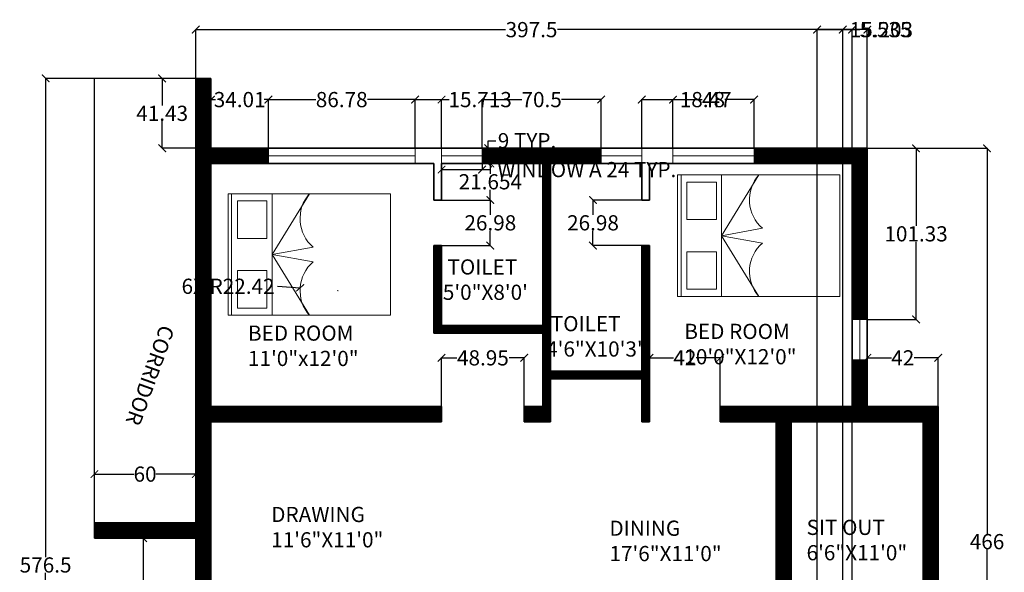
# Model space of a CAD drawing. Units: inches. Extents: x -124 to 468, y -83 to 563.
# Tile 3 of 3: x -124 to 459, y 235 to 563. Entities that reach past the tile are written whole.
import ezdxf

# ---------------------------------------------------------------- set-up
doc = ezdxf.new("R2010")
doc.units = ezdxf.units.IN
doc.header["$MEASUREMENT"] = 0
for name, color, linetype, lineweight in [('A-ANNO-DIMS', 2, 'Continuous', 18), ('A-AREA-IDEN', 7, 'Continuous', 18), ('A-FLOR', 8, 'Continuous', 25)]:
    doc.layers.add(name, color=color, linetype=linetype, lineweight=lineweight)
for name, color, linetype, lineweight, true_color in [('A-FURN', 37, 'Continuous', 18, 0x7c5b46), ('A-GLAZ', 145, 'Continuous', 18, 0x2a88b7), ('A-WALL', 149, 'Continuous', 35, 0x414448), ('A-WALL-PATT', 251, 'Continuous', 13, 0x585a5e)]:
    doc.layers.add(name, color=color, linetype=linetype, lineweight=lineweight, true_color=true_color)
doc.styles.get("Standard").update_dxf_attribs({"font": 'arial.ttf'})
doc.dimstyles.get("Standard").update_dxf_attribs({"dimtxt": 9, "dimasz": 4.5, "dimexe": 0.18, "dimexo": 0.0625, "dimgap": 0.09, "dimtad": 0, "dimtih": 1, "dimtoh": 1, "dimdec": 1, "dimzin": 0, "dimdsep": 46, "dimlunit": 4, "dimtxsty": 'Standard', "dimblk": 'ARCHTICK', "dimcen": 0.09, "dimadec": 0, "dimazin": 0, "dimtfac": 1, "dimtdec": 1, "dimtofl": 0, "dimtmove": 0, "dimatfit": 3, "dimfxl": 1, "dimtolj": 1, "dimtzin": 0, "dimarcsym": 0})

# ---------------------------------------------------------------- blocks, each defined once
blk = doc.blocks.new('BED-DOUBLE')
for p, q in [((0, 0), (0, 72)), ((0, 72), (96, 72)), ((2, 0), (2, 72)), ((26, 0), (26, 72)), ((48, 72), (26, 36)), ((96, 72), (96, 0)), ((26, 36), (50.21, 40.36)), ((26, 36), (48, 0)), ((26, 36), (50.21, 31.64)), ((50.21, 31.64), (26, 36)), ((96, 0), (0, 0))]:
    blk.add_line(p, q)
for points in [[(5.47, 67.74), (5.47, 45.52), (22.92, 45.52), (22.92, 67.74)], [(5.47, 4.26), (5.47, 26.48), (22.92, 26.48), (22.92, 4.26)]]:
    blk.add_lwpolyline(points, close=True)
for centre, start, end in [((64.91, 57.28), 138.97274, 229.00257), ((64.91, 14.72), 130.99743, 221.02726)]:
    blk.add_arc(centre, 22.42, start, end)
blk = doc.blocks.new('WIN-24IN')
for p, q in [((0, 0), (0, 9)), ((24, 0), (24, 9)), ((0, 4.5), (24, 4.5))]:
    blk.add_line(p, q)
blk = doc.blocks.new('_ArchTick')
at = {"color": 0, "linetype": 'ByBlock', "const_width": 0.15}
blk.add_lwpolyline([(-0.5, -0.5), (0.5, 0.5)], dxfattribs=at)
blk = doc.blocks.new('*D8')
at = {"layer": 'A-ANNO-DIMS', "color": 0, "lineweight": -2, "transparency": 16777216}
for p, q in [((125.98, 477.33), (125.98, 473.61)), ((125.98, 473.79), (149.98, 473.79)), ((149.98, 477.33), (149.98, 473.61)), ((149.98, 473.79), (154.48, 473.79))]:
    blk.add_line(p, q, dxfattribs=at)
at = {"layer": 'Defpoints', "color": 0, "transparency": 16777216}
for p in [(125.98, 477.39), (149.98, 477.39), (149.98, 473.79)]:
    blk.add_point(p, dxfattribs=at)
at = {"layer": 'A-ANNO-DIMS', "color": 0, "lineweight": -2, "transparency": 16777216, "xscale": 4.5, "yscale": 4.5, "zscale": 4.5, "rotation": 180}
blk.add_blockref('_ArchTick', (125.98, 473.79), dxfattribs=at)
at = {"layer": 'A-ANNO-DIMS', "color": 0, "lineweight": -2, "transparency": 16777216, "xscale": 4.5, "yscale": 4.5, "zscale": 4.5}
blk.add_blockref('_ArchTick', (149.98, 473.79), dxfattribs=at)
at = {"layer": 'A-ANNO-DIMS', "color": 0, "transparency": 16777216, "insert": (211.92, 473.79), "char_height": 9, "attachment_point": 5}
blk.add_mtext('\\A1;WINDOW A 24 TYP.', dxfattribs=at)
blk = doc.blocks.new('*D9')
at = {"layer": 'A-ANNO-DIMS', "color": 0, "lineweight": -2, "transparency": 16777216}
for p, q in [((153.58, 486.39), (153.58, 490.89)), ((153.58, 490.89), (158.08, 490.89)), ((150.04, 486.39), (153.76, 486.39)), ((153.58, 477.39), (153.58, 486.39)), ((150.04, 477.39), (153.76, 477.39))]:
    blk.add_line(p, q, dxfattribs=at)
at = {"layer": 'Defpoints', "color": 0, "transparency": 16777216}
for p in [(149.98, 486.39), (153.58, 486.39), (149.98, 477.39)]:
    blk.add_point(p, dxfattribs=at)
at = {"layer": 'A-ANNO-DIMS', "color": 0, "lineweight": -2, "transparency": 16777216, "xscale": 4.5, "yscale": 4.5, "zscale": 4.5}
for p, rotation in [((153.58, 486.39), 90), ((153.58, 477.39), 270)]:
    blk.add_blockref('_ArchTick', p, dxfattribs=dict(at, rotation=rotation))
at = {"layer": 'A-ANNO-DIMS', "color": 0, "transparency": 16777216, "insert": (176.57, 490.89), "char_height": 9, "attachment_point": 5}
blk.add_mtext('\\A1;9 TYP.', dxfattribs=at)
blk = doc.blocks.new('*D15')
at = {"layer": 'A-ANNO-DIMS', "color": 0, "lineweight": -2, "transparency": 16777216}
for p, q in [((-19.59, 527.82), (-108.57, 527.82)), ((-108.39, 527.82), (-108.39, 244.25)), ((-108.39, -48.69), (-108.39, 234.88)), ((-19.59, -48.69), (-108.57, -48.69))]:
    blk.add_line(p, q, dxfattribs=at)
at = {"layer": 'Defpoints', "color": 0, "transparency": 16777216}
for p in [(-108.39, 527.82), (-19.52, 527.82), (-19.52, -48.69)]:
    blk.add_point(p, dxfattribs=at)
at = {"layer": 'A-ANNO-DIMS', "color": 0, "lineweight": -2, "transparency": 16777216, "xscale": 4.5, "yscale": 4.5, "zscale": 4.5}
for p, rotation in [((-108.39, 527.82), 90), ((-108.39, -48.69), 270)]:
    blk.add_blockref('_ArchTick', p, dxfattribs=dict(at, rotation=rotation))
at = {"layer": 'A-ANNO-DIMS', "color": 0, "transparency": 16777216, "insert": (-108.39, 239.57), "char_height": 9, "attachment_point": 5}
blk.add_mtext('\\A1;576.5', dxfattribs=at)
blk = doc.blocks.new('*D16')
at = {"layer": 'A-ANNO-DIMS', "color": 0, "lineweight": -2, "transparency": 16777216}
for p, q in [((-19.52, 527.89), (-19.52, 556.87)), ((-19.52, 556.69), (163.92, 556.69)), ((377.98, 556.69), (194.53, 556.69)), ((377.98, 486.46), (377.98, 556.87))]:
    blk.add_line(p, q, dxfattribs=at)
at = {"layer": 'Defpoints', "color": 0, "transparency": 16777216}
for p in [(377.98, 556.69), (-19.52, 527.82), (377.98, 486.39)]:
    blk.add_point(p, dxfattribs=at)
at = {"layer": 'A-ANNO-DIMS', "color": 0, "lineweight": -2, "transparency": 16777216, "xscale": 4.5, "yscale": 4.5, "zscale": 4.5, "rotation": 180}
blk.add_blockref('_ArchTick', (-19.52, 556.69), dxfattribs=at)
at = {"layer": 'A-ANNO-DIMS', "color": 0, "lineweight": -2, "transparency": 16777216, "xscale": 4.5, "yscale": 4.5, "zscale": 4.5}
blk.add_blockref('_ArchTick', (377.98, 556.69), dxfattribs=at)
at = {"layer": 'A-ANNO-DIMS', "color": 0, "transparency": 16777216, "insert": (179.23, 556.69), "char_height": 9, "attachment_point": 5}
blk.add_mtext('\\A1;397.5', dxfattribs=at)
blk = doc.blocks.new('*D17')
at = {"layer": 'A-ANNO-DIMS', "color": 0, "lineweight": -2, "transparency": 16777216}
for p, q in [((378.04, 486.39), (449.02, 486.39)), ((448.84, 486.39), (448.84, 258.08)), ((448.84, 20.39), (448.84, 248.71)), ((378.04, 20.39), (449.02, 20.39))]:
    blk.add_line(p, q, dxfattribs=at)
at = {"layer": 'Defpoints', "color": 0, "transparency": 16777216}
for p in [(377.98, 486.39), (448.84, 486.39), (377.98, 20.39)]:
    blk.add_point(p, dxfattribs=at)
at = {"layer": 'A-ANNO-DIMS', "color": 0, "lineweight": -2, "transparency": 16777216, "xscale": 4.5, "yscale": 4.5, "zscale": 4.5}
for p, rotation in [((448.84, 486.39), 90), ((448.84, 20.39), 270)]:
    blk.add_blockref('_ArchTick', p, dxfattribs=dict(at, rotation=rotation))
at = {"layer": 'A-ANNO-DIMS', "color": 0, "transparency": 16777216, "insert": (448.84, 253.39), "char_height": 9, "attachment_point": 5}
blk.add_mtext('\\A1;466', dxfattribs=at)
blk = doc.blocks.new('*D18')
at = {"layer": 'A-ANNO-DIMS', "color": 0, "lineweight": -2, "transparency": 16777216}
for p, q in [((-10.59, 527.82), (-39.57, 527.82)), ((-39.39, 527.82), (-39.39, 511.8)), ((-39.39, 486.39), (-39.39, 502.42)), ((-10.59, 486.39), (-39.57, 486.39))]:
    blk.add_line(p, q, dxfattribs=at)
at = {"layer": 'Defpoints', "color": 0, "transparency": 16777216}
for p in [(-39.39, 527.82), (-10.52, 527.82), (-10.52, 486.39)]:
    blk.add_point(p, dxfattribs=at)
at = {"layer": 'A-ANNO-DIMS', "color": 0, "lineweight": -2, "transparency": 16777216, "xscale": 4.5, "yscale": 4.5, "zscale": 4.5}
for p, rotation in [((-39.39, 527.82), 90), ((-39.39, 486.39), 270)]:
    blk.add_blockref('_ArchTick', p, dxfattribs=dict(at, rotation=rotation))
at = {"layer": 'A-ANNO-DIMS', "color": 0, "transparency": 16777216, "insert": (-39.39, 507.11), "char_height": 9, "attachment_point": 5}
blk.add_mtext('\\A1;41.43', dxfattribs=at)
blk = doc.blocks.new('*D19')
at = {"layer": 'A-ANNO-DIMS', "color": 0, "lineweight": -2, "transparency": 16777216}
for p, q in [((-79.52, 264.59), (-79.52, 293.57)), ((-79.52, 293.39), (-56.07, 293.39)), ((-19.52, 293.39), (-42.98, 293.39)), ((-19.52, 264.59), (-19.52, 293.57))]:
    blk.add_line(p, q, dxfattribs=at)
at = {"layer": 'Defpoints', "color": 0, "transparency": 16777216}
for p in [(-19.52, 293.39), (-79.52, 264.53), (-19.52, 264.53)]:
    blk.add_point(p, dxfattribs=at)
at = {"layer": 'A-ANNO-DIMS', "color": 0, "lineweight": -2, "transparency": 16777216, "xscale": 4.5, "yscale": 4.5, "zscale": 4.5, "rotation": 180}
blk.add_blockref('_ArchTick', (-79.52, 293.39), dxfattribs=at)
at = {"layer": 'A-ANNO-DIMS', "color": 0, "lineweight": -2, "transparency": 16777216, "xscale": 4.5, "yscale": 4.5, "zscale": 4.5}
blk.add_blockref('_ArchTick', (-19.52, 293.39), dxfattribs=at)
at = {"layer": 'A-ANNO-DIMS', "color": 0, "transparency": 16777216, "insert": (-49.52, 293.39), "char_height": 9, "attachment_point": 5}
blk.add_mtext('\\A1;60', dxfattribs=at)
blk = doc.blocks.new('*D20')
at = {"layer": 'A-ANNO-DIMS', "color": 0, "lineweight": -2, "transparency": 16777216}
for p, q in [((377.98, 333.46), (377.98, 362.44)), ((377.98, 362.26), (392.31, 362.26)), ((419.98, 362.26), (405.65, 362.26)), ((419.98, 333.46), (419.98, 362.44))]:
    blk.add_line(p, q, dxfattribs=at)
at = {"layer": 'Defpoints', "color": 0, "transparency": 16777216}
for p in [(419.98, 362.26), (377.98, 333.39), (419.98, 333.39)]:
    blk.add_point(p, dxfattribs=at)
at = {"layer": 'A-ANNO-DIMS', "color": 0, "lineweight": -2, "transparency": 16777216, "xscale": 4.5, "yscale": 4.5, "zscale": 4.5, "rotation": 180}
blk.add_blockref('_ArchTick', (377.98, 362.26), dxfattribs=at)
at = {"layer": 'A-ANNO-DIMS', "color": 0, "lineweight": -2, "transparency": 16777216, "xscale": 4.5, "yscale": 4.5, "zscale": 4.5}
blk.add_blockref('_ArchTick', (419.98, 362.26), dxfattribs=at)
at = {"layer": 'A-ANNO-DIMS', "color": 0, "transparency": 16777216, "insert": (398.98, 362.26), "char_height": 9, "attachment_point": 5}
blk.add_mtext('\\A1;42', dxfattribs=at)
blk = doc.blocks.new('*D22')
at = {"layer": 'A-ANNO-DIMS', "color": 0, "lineweight": -2, "transparency": 16777216}
for p, q in [((-10.52, 486.46), (-10.52, 515.44)), ((-10.52, 515.26), (-7.92, 515.26)), ((23.48, 515.26), (20.88, 515.26)), ((23.48, 486.46), (23.48, 515.44))]:
    blk.add_line(p, q, dxfattribs=at)
at = {"layer": 'Defpoints', "color": 0, "transparency": 16777216}
for p in [(23.48, 515.26), (-10.52, 486.39), (23.48, 486.39)]:
    blk.add_point(p, dxfattribs=at)
at = {"layer": 'A-ANNO-DIMS', "color": 0, "lineweight": -2, "transparency": 16777216, "xscale": 4.5, "yscale": 4.5, "zscale": 4.5, "rotation": 180}
blk.add_blockref('_ArchTick', (-10.52, 515.26), dxfattribs=at)
at = {"layer": 'A-ANNO-DIMS', "color": 0, "lineweight": -2, "transparency": 16777216, "xscale": 4.5, "yscale": 4.5, "zscale": 4.5}
blk.add_blockref('_ArchTick', (23.48, 515.26), dxfattribs=at)
at = {"layer": 'A-ANNO-DIMS', "color": 0, "transparency": 16777216, "insert": (6.48, 515.26), "char_height": 9, "attachment_point": 5}
blk.add_mtext('\\A1;34.01', dxfattribs=at)
blk = doc.blocks.new('*D23')
at = {"layer": 'A-ANNO-DIMS', "color": 0, "lineweight": -2, "transparency": 16777216}
for p, q in [((23.48, 486.46), (23.48, 515.44)), ((23.48, 515.26), (51.58, 515.26)), ((110.26, 515.26), (82.16, 515.26)), ((110.26, 486.46), (110.26, 515.44))]:
    blk.add_line(p, q, dxfattribs=at)
at = {"layer": 'Defpoints', "color": 0, "transparency": 16777216}
for p in [(110.26, 515.26), (23.48, 486.39), (110.26, 486.39)]:
    blk.add_point(p, dxfattribs=at)
at = {"layer": 'A-ANNO-DIMS', "color": 0, "lineweight": -2, "transparency": 16777216, "xscale": 4.5, "yscale": 4.5, "zscale": 4.5, "rotation": 180}
blk.add_blockref('_ArchTick', (23.48, 515.26), dxfattribs=at)
at = {"layer": 'A-ANNO-DIMS', "color": 0, "lineweight": -2, "transparency": 16777216, "xscale": 4.5, "yscale": 4.5, "zscale": 4.5}
blk.add_blockref('_ArchTick', (110.26, 515.26), dxfattribs=at)
at = {"layer": 'A-ANNO-DIMS', "color": 0, "transparency": 16777216, "insert": (66.87, 515.26), "char_height": 9, "attachment_point": 5}
blk.add_mtext('\\A1;86.78', dxfattribs=at)
blk = doc.blocks.new('*D24')
at = {"layer": 'A-ANNO-DIMS', "color": 0, "lineweight": -2, "transparency": 16777216}
for p, q in [((110.26, 486.46), (110.26, 515.44)), ((110.26, 515.26), (125.98, 515.26)), ((125.98, 486.46), (125.98, 515.44)), ((125.98, 515.26), (130.48, 515.26))]:
    blk.add_line(p, q, dxfattribs=at)
at = {"layer": 'Defpoints', "color": 0, "transparency": 16777216}
for p in [(125.98, 515.26), (110.26, 486.39), (125.98, 486.39)]:
    blk.add_point(p, dxfattribs=at)
at = {"layer": 'A-ANNO-DIMS', "color": 0, "lineweight": -2, "transparency": 16777216, "xscale": 4.5, "yscale": 4.5, "zscale": 4.5, "rotation": 180}
blk.add_blockref('_ArchTick', (110.26, 515.26), dxfattribs=at)
at = {"layer": 'A-ANNO-DIMS', "color": 0, "lineweight": -2, "transparency": 16777216, "xscale": 4.5, "yscale": 4.5, "zscale": 4.5}
blk.add_blockref('_ArchTick', (125.98, 515.26), dxfattribs=at)
at = {"layer": 'A-ANNO-DIMS', "color": 0, "transparency": 16777216, "insert": (148.82, 515.26), "char_height": 9, "attachment_point": 5}
blk.add_mtext('\\A1;15.713', dxfattribs=at)
blk = doc.blocks.new('*D25')
at = {"layer": 'A-ANNO-DIMS', "color": 0, "lineweight": -2, "transparency": 16777216}
for p, q in [((149.98, 486.46), (149.98, 515.44)), ((149.98, 515.26), (173.45, 515.26)), ((220.48, 515.26), (197, 515.26)), ((220.48, 486.46), (220.48, 515.44))]:
    blk.add_line(p, q, dxfattribs=at)
at = {"layer": 'Defpoints', "color": 0, "transparency": 16777216}
for p in [(220.48, 515.26), (149.98, 486.39), (220.48, 486.39)]:
    blk.add_point(p, dxfattribs=at)
at = {"layer": 'A-ANNO-DIMS', "color": 0, "lineweight": -2, "transparency": 16777216, "xscale": 4.5, "yscale": 4.5, "zscale": 4.5, "rotation": 180}
blk.add_blockref('_ArchTick', (149.98, 515.26), dxfattribs=at)
at = {"layer": 'A-ANNO-DIMS', "color": 0, "lineweight": -2, "transparency": 16777216, "xscale": 4.5, "yscale": 4.5, "zscale": 4.5}
blk.add_blockref('_ArchTick', (220.48, 515.26), dxfattribs=at)
at = {"layer": 'A-ANNO-DIMS', "color": 0, "transparency": 16777216, "insert": (185.23, 515.26), "char_height": 9, "attachment_point": 5}
blk.add_mtext('\\A1;70.5', dxfattribs=at)
blk = doc.blocks.new('*D26')
at = {"layer": 'A-ANNO-DIMS', "color": 0, "lineweight": -2, "transparency": 16777216}
for p, q in [((244.48, 486.46), (244.48, 515.44)), ((244.48, 515.26), (262.95, 515.26)), ((262.95, 486.46), (262.95, 515.44)), ((262.95, 515.26), (267.45, 515.26))]:
    blk.add_line(p, q, dxfattribs=at)
at = {"layer": 'Defpoints', "color": 0, "transparency": 16777216}
for p in [(262.95, 515.26), (244.48, 486.39), (262.95, 486.39)]:
    blk.add_point(p, dxfattribs=at)
at = {"layer": 'A-ANNO-DIMS', "color": 0, "lineweight": -2, "transparency": 16777216, "xscale": 4.5, "yscale": 4.5, "zscale": 4.5, "rotation": 180}
blk.add_blockref('_ArchTick', (244.48, 515.26), dxfattribs=at)
at = {"layer": 'A-ANNO-DIMS', "color": 0, "lineweight": -2, "transparency": 16777216, "xscale": 4.5, "yscale": 4.5, "zscale": 4.5}
blk.add_blockref('_ArchTick', (262.95, 515.26), dxfattribs=at)
at = {"layer": 'A-ANNO-DIMS', "color": 0, "transparency": 16777216, "insert": (282.3, 515.26), "char_height": 9, "attachment_point": 5}
blk.add_mtext('\\A1;18.47', dxfattribs=at)
blk = doc.blocks.new('*D27')
at = {"layer": 'A-ANNO-DIMS', "color": 0, "lineweight": -2, "transparency": 16777216}
for p, q in [((262.95, 486.46), (262.95, 515.44)), ((262.95, 515.26), (280.22, 515.26)), ((310.95, 515.26), (293.67, 515.26)), ((310.95, 486.46), (310.95, 515.44))]:
    blk.add_line(p, q, dxfattribs=at)
at = {"layer": 'Defpoints', "color": 0, "transparency": 16777216}
for p in [(310.95, 515.26), (262.95, 486.39), (310.95, 486.39)]:
    blk.add_point(p, dxfattribs=at)
at = {"layer": 'A-ANNO-DIMS', "color": 0, "lineweight": -2, "transparency": 16777216, "xscale": 4.5, "yscale": 4.5, "zscale": 4.5, "rotation": 180}
blk.add_blockref('_ArchTick', (262.95, 515.26), dxfattribs=at)
at = {"layer": 'A-ANNO-DIMS', "color": 0, "lineweight": -2, "transparency": 16777216, "xscale": 4.5, "yscale": 4.5, "zscale": 4.5}
blk.add_blockref('_ArchTick', (310.95, 515.26), dxfattribs=at)
at = {"layer": 'A-ANNO-DIMS', "color": 0, "transparency": 16777216, "insert": (286.95, 515.26), "char_height": 9, "attachment_point": 5}
blk.add_mtext('\\A1;48', dxfattribs=at)
blk = doc.blocks.new('*D33')
at = {"layer": 'A-ANNO-DIMS', "color": 0, "lineweight": -2, "transparency": 16777216}
for p, q in [((378.04, 486.39), (407.02, 486.39)), ((406.84, 486.39), (406.84, 440.42)), ((406.84, 385.07), (406.84, 431.04)), ((378.04, 385.07), (407.02, 385.07))]:
    blk.add_line(p, q, dxfattribs=at)
at = {"layer": 'Defpoints', "color": 0, "transparency": 16777216}
for p in [(377.98, 486.39), (377.98, 385.07), (406.84, 385.07)]:
    blk.add_point(p, dxfattribs=at)
at = {"layer": 'A-ANNO-DIMS', "color": 0, "lineweight": -2, "transparency": 16777216, "xscale": 4.5, "yscale": 4.5, "zscale": 4.5}
for p, rotation in [((406.84, 486.39), 90), ((406.84, 385.07), 270)]:
    blk.add_blockref('_ArchTick', p, dxfattribs=dict(at, rotation=rotation))
at = {"layer": 'A-ANNO-DIMS', "color": 0, "transparency": 16777216, "insert": (406.84, 435.73), "char_height": 9, "attachment_point": 5}
blk.add_mtext('\\A1;101.33', dxfattribs=at)
blk = doc.blocks.new('*D36')
at = {"layer": 'A-ANNO-DIMS', "color": 0, "lineweight": -2, "transparency": 16777216}
for p, q in [((-79.46, 255.53), (-50.48, 255.53)), ((-50.66, 255.53), (-50.66, 210.64)), ((-50.66, 156.37), (-50.66, 201.27)), ((-79.46, 156.37), (-50.48, 156.37))]:
    blk.add_line(p, q, dxfattribs=at)
at = {"layer": 'Defpoints', "color": 0, "transparency": 16777216}
for p in [(-79.52, 255.53), (-79.52, 156.37), (-50.66, 156.37)]:
    blk.add_point(p, dxfattribs=at)
at = {"layer": 'A-ANNO-DIMS', "color": 0, "lineweight": -2, "transparency": 16777216, "xscale": 4.5, "yscale": 4.5, "zscale": 4.5}
for p, rotation in [((-50.66, 255.53), 90), ((-50.66, 156.37), 270)]:
    blk.add_blockref('_ArchTick', p, dxfattribs=dict(at, rotation=rotation))
at = {"layer": 'A-ANNO-DIMS', "color": 0, "transparency": 16777216, "insert": (-50.66, 205.95), "char_height": 9, "attachment_point": 5}
blk.add_mtext('\\A1;99.15', dxfattribs=at)
blk = doc.blocks.new('*D38')
at = {"layer": 'A-ANNO-DIMS', "color": 0, "lineweight": -2, "transparency": 16777216}
for p, q in [((125.98, 333.46), (125.98, 362.44)), ((125.98, 362.26), (134.96, 362.26)), ((174.93, 362.26), (165.94, 362.26)), ((174.93, 333.46), (174.93, 362.44))]:
    blk.add_line(p, q, dxfattribs=at)
at = {"layer": 'Defpoints', "color": 0, "transparency": 16777216}
for p in [(174.93, 362.26), (125.98, 333.39), (174.93, 333.39)]:
    blk.add_point(p, dxfattribs=at)
at = {"layer": 'A-ANNO-DIMS', "color": 0, "lineweight": -2, "transparency": 16777216, "xscale": 4.5, "yscale": 4.5, "zscale": 4.5, "rotation": 180}
blk.add_blockref('_ArchTick', (125.98, 362.26), dxfattribs=at)
at = {"layer": 'A-ANNO-DIMS', "color": 0, "lineweight": -2, "transparency": 16777216, "xscale": 4.5, "yscale": 4.5, "zscale": 4.5}
blk.add_blockref('_ArchTick', (174.93, 362.26), dxfattribs=at)
at = {"layer": 'A-ANNO-DIMS', "color": 0, "transparency": 16777216, "insert": (150.45, 362.26), "char_height": 9, "attachment_point": 5}
blk.add_mtext('\\A1;48.95', dxfattribs=at)
blk = doc.blocks.new('*D39')
at = {"layer": 'A-ANNO-DIMS', "color": 0, "lineweight": -2, "transparency": 16777216}
for p, q in [((248.98, 333.46), (248.98, 362.44)), ((248.98, 362.26), (263.31, 362.26)), ((290.98, 362.26), (276.65, 362.26)), ((290.98, 333.46), (290.98, 362.44))]:
    blk.add_line(p, q, dxfattribs=at)
at = {"layer": 'Defpoints', "color": 0, "transparency": 16777216}
for p in [(290.98, 362.26), (248.98, 333.39), (290.98, 333.39)]:
    blk.add_point(p, dxfattribs=at)
at = {"layer": 'A-ANNO-DIMS', "color": 0, "lineweight": -2, "transparency": 16777216, "xscale": 4.5, "yscale": 4.5, "zscale": 4.5, "rotation": 180}
blk.add_blockref('_ArchTick', (248.98, 362.26), dxfattribs=at)
at = {"layer": 'A-ANNO-DIMS', "color": 0, "lineweight": -2, "transparency": 16777216, "xscale": 4.5, "yscale": 4.5, "zscale": 4.5}
blk.add_blockref('_ArchTick', (290.98, 362.26), dxfattribs=at)
at = {"layer": 'A-ANNO-DIMS', "color": 0, "transparency": 16777216, "insert": (269.98, 362.26), "char_height": 9, "attachment_point": 5}
blk.add_mtext('\\A1;42', dxfattribs=at)
blk = doc.blocks.new('*D42')
at = {"layer": 'A-ANNO-DIMS', "color": 0, "lineweight": -2, "transparency": 16777216}
for p, q in [((126.04, 455.74), (155.02, 455.74)), ((154.84, 455.74), (154.84, 446.93)), ((154.84, 428.76), (154.84, 437.56)), ((126.04, 428.76), (155.02, 428.76))]:
    blk.add_line(p, q, dxfattribs=at)
at = {"layer": 'Defpoints', "color": 0, "transparency": 16777216}
for p in [(125.98, 455.74), (125.98, 428.76), (154.84, 428.76)]:
    blk.add_point(p, dxfattribs=at)
at = {"layer": 'A-ANNO-DIMS', "color": 0, "lineweight": -2, "transparency": 16777216, "xscale": 4.5, "yscale": 4.5, "zscale": 4.5}
for p, rotation in [((154.84, 455.74), 90), ((154.84, 428.76), 270)]:
    blk.add_blockref('_ArchTick', p, dxfattribs=dict(at, rotation=rotation))
at = {"layer": 'A-ANNO-DIMS', "color": 0, "transparency": 16777216, "insert": (154.84, 442.25), "char_height": 9, "attachment_point": 5}
blk.add_mtext('\\A1;26.98', dxfattribs=at)
blk = doc.blocks.new('*D43')
at = {"layer": 'A-ANNO-DIMS', "color": 0, "lineweight": -2, "transparency": 16777216}
for p, q in [((244.41, 455.74), (215.43, 455.74)), ((215.61, 455.74), (215.61, 446.93)), ((215.61, 428.76), (215.61, 437.56)), ((244.41, 428.76), (215.43, 428.76))]:
    blk.add_line(p, q, dxfattribs=at)
at = {"layer": 'Defpoints', "color": 0, "transparency": 16777216}
for p in [(215.61, 455.74), (244.48, 455.74), (244.48, 428.76)]:
    blk.add_point(p, dxfattribs=at)
at = {"layer": 'A-ANNO-DIMS', "color": 0, "lineweight": -2, "transparency": 16777216, "xscale": 4.5, "yscale": 4.5, "zscale": 4.5}
for p, rotation in [((215.61, 455.74), 90), ((215.61, 428.76), 270)]:
    blk.add_blockref('_ArchTick', p, dxfattribs=dict(at, rotation=rotation))
at = {"layer": 'A-ANNO-DIMS', "color": 0, "transparency": 16777216, "insert": (215.61, 442.25), "char_height": 9, "attachment_point": 5}
blk.add_mtext('\\A1;26.98', dxfattribs=at)
blk = doc.blocks.new('*D44')
at = {"layer": 'A-ANNO-DIMS', "color": 0, "lineweight": -2, "transparency": 16777216}
for p, q in [((126.04, 477.39), (155.02, 477.39)), ((154.84, 477.39), (154.84, 471.25)), ((154.84, 455.74), (154.84, 461.88)), ((126.04, 455.74), (155.02, 455.74))]:
    blk.add_line(p, q, dxfattribs=at)
at = {"layer": 'Defpoints', "color": 0, "transparency": 16777216}
for p in [(125.98, 477.39), (125.98, 455.74), (154.84, 455.74)]:
    blk.add_point(p, dxfattribs=at)
at = {"layer": 'A-ANNO-DIMS', "color": 0, "lineweight": -2, "transparency": 16777216, "xscale": 4.5, "yscale": 4.5, "zscale": 4.5}
for p, rotation in [((154.84, 477.39), 90), ((154.84, 455.74), 270)]:
    blk.add_blockref('_ArchTick', p, dxfattribs=dict(at, rotation=rotation))
at = {"layer": 'A-ANNO-DIMS', "color": 0, "transparency": 16777216, "insert": (154.84, 466.57), "char_height": 9, "attachment_point": 5}
blk.add_mtext('\\A1;21.654', dxfattribs=at)
blk = doc.blocks.new('*D56')
at = {"layer": 'A-ANNO-DIMS', "color": 0, "lineweight": -2, "transparency": 16777216}
for p, q in [((348.24, 156.86), (348.24, 556.87)), ((348.24, 556.69), (363.44, 556.69)), ((363.44, 156.86), (363.44, 556.87)), ((363.44, 556.69), (367.94, 556.69))]:
    blk.add_line(p, q, dxfattribs=at)
at = {"layer": 'Defpoints', "color": 0, "transparency": 16777216}
for p in [(363.44, 556.69), (348.24, 156.8), (363.44, 156.8)]:
    blk.add_point(p, dxfattribs=at)
at = {"layer": 'A-ANNO-DIMS', "color": 0, "lineweight": -2, "transparency": 16777216, "xscale": 4.5, "yscale": 4.5, "zscale": 4.5, "rotation": 180}
blk.add_blockref('_ArchTick', (348.24, 556.69), dxfattribs=at)
at = {"layer": 'A-ANNO-DIMS', "color": 0, "lineweight": -2, "transparency": 16777216, "xscale": 4.5, "yscale": 4.5, "zscale": 4.5}
blk.add_blockref('_ArchTick', (363.44, 556.69), dxfattribs=at)
at = {"layer": 'A-ANNO-DIMS', "color": 0, "transparency": 16777216, "insert": (386.29, 556.69), "char_height": 9, "attachment_point": 5}
blk.add_mtext('\\A1;15.203', dxfattribs=at)
blk = doc.blocks.new('*D59')
at = {"layer": 'A-ANNO-DIMS', "color": 0, "lineweight": -2, "transparency": 16777216}
for p, q in [((363.44, 156.86), (363.44, 556.87)), ((363.44, 556.69), (368.98, 556.69)), ((368.98, 183.46), (368.98, 556.87)), ((368.98, 556.69), (373.48, 556.69))]:
    blk.add_line(p, q, dxfattribs=at)
at = {"layer": 'Defpoints', "color": 0, "transparency": 16777216}
for p in [(368.98, 556.69), (368.98, 183.39), (363.44, 156.8)]:
    blk.add_point(p, dxfattribs=at)
at = {"layer": 'A-ANNO-DIMS', "color": 0, "lineweight": -2, "transparency": 16777216, "xscale": 4.5, "yscale": 4.5, "zscale": 4.5, "rotation": 180}
blk.add_blockref('_ArchTick', (363.44, 556.69), dxfattribs=at)
at = {"layer": 'A-ANNO-DIMS', "color": 0, "lineweight": -2, "transparency": 16777216, "xscale": 4.5, "yscale": 4.5, "zscale": 4.5}
blk.add_blockref('_ArchTick', (368.98, 556.69), dxfattribs=at)
at = {"layer": 'A-ANNO-DIMS', "color": 0, "transparency": 16777216, "insert": (388.79, 556.69), "char_height": 9, "attachment_point": 5}
blk.add_mtext('\\A1;5.535', dxfattribs=at)
blk = doc.blocks.new('*D62')
at = {"layer": 'A-ANNO-DIMS', "color": 0, "lineweight": -2, "transparency": 16777216}
for p, q in [((28.84, 404.66), (42.26, 403.73)), ((64.54, 402.17), (64.72, 402.17)), ((64.63, 402.08), (64.63, 402.26))]:
    blk.add_line(p, q, dxfattribs=at)
at = {"layer": 'Defpoints', "color": 0, "transparency": 16777216}
for p in [(42.26, 403.73), (64.63, 402.17)]:
    blk.add_point(p, dxfattribs=at)
at = {"layer": 'A-ANNO-DIMS', "color": 0, "lineweight": -2, "transparency": 16777216, "xscale": 4.5, "yscale": 4.5, "zscale": 4.5, "rotation": 356.0116510722241}
blk.add_blockref('_ArchTick', (42.26, 403.73), dxfattribs=at)
at = {"layer": 'A-ANNO-DIMS', "color": 0, "transparency": 16777216, "insert": (-0.39, 404.66), "char_height": 9, "attachment_point": 5}
blk.add_mtext('\\A1;6X R22.42', dxfattribs=at)

msp = doc.modelspace()

# ---------------------------------------------------------------- hatches: boundary and pattern name
at = {"layer": 'A-WALL-PATT'}
h = msp.add_hatch(dxfattribs=at)
h.set_pattern_fill('ANSI31', color=256)
h.set_pattern_definition([(45, (-392.07623, 0), (-0.088388348, 0.088388348), [])])
h.paths.add_polyline_path([(377.9763, 141.7862), (377.9763, 183.3929), (419.9763, 183.3929), (419.9763, 192.3929), (419.9763, 324.3929), (419.9763, 333.3929), (377.9763, 333.3929), (377.9763, 361.0673), (368.9763, 361.0673), (368.9763, 333.3929), (290.9763, 333.3929), (290.9763, 324.3929), (323.9763, 324.3929), (323.9763, 192.3929), (323.9763, 183.3929), (368.9763, 183.3929), (368.9763, 141.7862), (368.9763, 29.3929), (343.3064, 29.3929), (343.3064, 20.3929), (377.9763, 20.3929)])
h.paths.add_polyline_path([(368.9763, 192.3929), (332.9763, 192.3929), (332.9763, 324.3929), (368.9763, 324.3929), (410.9763, 324.3929), (410.9763, 192.3929)], flags=16)
h.paths.add_polyline_path([(215.9763, 29.3929), (179.9763, 29.3929), (179.9763, 75.2245), (175.4763, 75.2245), (175.4763, 29.3929), (167.489, 29.3929), (167.489, 20.3929), (215.9763, 20.3929)])
h.paths.add_polyline_path([(266.8777, 29.3929), (244.4763, 29.3929), (244.4763, 141.7862), (244.4763, 183.3929), (257.421, 183.3929), (257.421, 192.3929), (170.9763, 192.3929), (170.9763, 183.3929), (175.4763, 183.3929), (175.4763, 141.7862), (175.4763, 106.8322), (179.9763, 106.8322), (179.9763, 141.7862), (179.9763, 183.3929), (239.9763, 183.3929), (239.9763, 141.7862), (239.9763, 29.3929), (239.9763, 20.3929), (266.8777, 20.3929)])
h.paths.add_polyline_path([(131.489, 29.3929), (62.8565, 29.3929), (62.8565, 20.3929), (131.489, 20.3929)])
h.paths.add_polyline_path([(26.8565, 29.3929), (-10.5237, 29.3929), (-10.5237, 141.7862), (-10.5237, 183.3929), (125.9763, 183.3929), (125.9763, 192.3929), (-10.5237, 192.3929), (-10.5237, 324.3929), (125.9763, 324.3929), (125.9763, 333.3929), (-10.5237, 333.3929), (-10.5237, 477.3929), (23.4837, 477.3929), (23.4837, 486.3929), (-10.5237, 486.3929), (-10.5237, 527.8228), (-19.5237, 527.8228), (-19.5237, 486.3929), (-19.5237, 264.528), (-79.5237, 264.528), (-79.5237, 255.528), (-19.5237, 255.528), (-19.5237, 156.3747), (-79.5237, 156.3747), (-79.5237, 147.3747), (-19.5237, 147.3747), (-19.5237, 141.7862), (-19.5237, -48.6869), (-10.5237, -48.6869), (-10.5237, 20.3929), (26.8565, 20.3929)])
h.paths.add_polyline_path([(220.4763, 486.3929), (149.9763, 486.3929), (149.9763, 477.3929), (185.9763, 477.3929), (185.9763, 381.3929), (125.9763, 381.3929), (125.9763, 428.759), (121.4763, 428.759), (121.4763, 376.8929), (125.9763, 376.8929), (185.9763, 376.8929), (185.9763, 333.3929), (174.9252, 333.3929), (174.9252, 324.3929), (190.4763, 324.3929), (190.4763, 333.3929), (190.4763, 349.8929), (244.4763, 349.8929), (244.4763, 333.3929), (244.4763, 324.3929), (248.9763, 324.3929), (248.9763, 333.3929), (248.9763, 428.759), (244.4763, 428.759), (244.4763, 354.3929), (190.4763, 354.3929), (190.4763, 477.3929), (220.4763, 477.3929)])
h.paths.add_polyline_path([(377.9763, 486.3929), (310.948, 486.3929), (310.948, 477.3929), (368.9763, 477.3929), (368.9763, 385.0673), (377.9763, 385.0673)])
h.paths.add_polyline_path([(339.1974, 237.2234), (400.8652, 237.2234), (400.8652, 270.8067), (339.1974, 270.8067)], flags=8)
h.paths.add_polyline_path([(182.8614, 357.8948), (247.9303, 357.8948), (247.9303, 391.478), (182.8614, 391.478)], flags=25)

# ---------------------------------------------------------------- linework, layer by layer
at = {"layer": 'A-FLOR'}
for p in [(-79.5237, 264.528), (-19.5237, 527.8228)]:
    msp.add_line(p, (-79.5237, 527.8228), dxfattribs=at)
at = {"layer": 'A-GLAZ'}
for p, q in [((23.4837, 486.3929), (23.4837, 477.3929)), ((110.2629, 486.3929), (110.2629, 477.3929)), ((262.948, 486.3929), (262.948, 477.3929)), ((310.948, 486.3929), (310.948, 477.3929)), ((23.4837, 481.8929), (110.2629, 481.8929)), ((262.948, 481.8929), (310.948, 481.8929))]:
    msp.add_line(p, q, dxfattribs=at)
at = {"layer": 'A-WALL'}
for p, q in [((-19.5237, 486.3929), (-19.5237, 527.8228)), ((-19.5237, 527.8228), (-10.5237, 527.8228)), ((-10.5237, 486.3929), (-10.5237, 527.8228)), ((-19.5237, 486.3929), (-19.5237, 264.528)), ((-10.5237, 486.3929), (377.9763, 486.3929)), ((377.9763, 486.3929), (377.9763, 333.3929)), ((-10.5237, 477.3929), (-10.5237, 333.3929)), ((-10.5237, 477.3929), (121.4763, 477.3929)), ((121.4763, 477.3929), (121.4763, 455.7385)), ((125.9763, 477.3929), (125.9763, 455.7385)), ((125.9763, 477.3929), (185.9763, 477.3929)), ((185.9763, 477.3929), (185.9763, 381.3929)), ((190.4763, 477.3929), (190.4763, 354.3929)), ((190.4763, 477.3929), (244.4763, 477.3929)), ((244.4763, 477.3929), (244.4763, 455.7385)), ((248.9763, 477.3929), (248.9763, 455.7385)), ((248.9763, 477.3929), (368.9763, 477.3929)), ((368.9763, 477.3929), (368.9763, 333.3929)), ((125.9763, 455.7385), (121.4763, 455.7385)), ((244.4763, 455.7385), (248.9763, 455.7385)), ((121.4763, 428.759), (121.4763, 376.8929)), ((125.9763, 428.759), (121.4763, 428.759)), ((125.9763, 428.759), (125.9763, 381.3929)), ((244.4763, 428.759), (248.9763, 428.759)), ((244.4763, 428.759), (244.4763, 354.3929)), ((248.9763, 428.759), (248.9763, 333.3929)), ((125.9763, 381.3929), (185.9763, 381.3929)), ((125.9763, 376.8929), (121.4763, 376.8929)), ((125.9763, 376.8929), (185.9763, 376.8929)), ((185.9763, 376.8929), (185.9763, 333.3929)), ((190.4763, 354.3929), (244.4763, 354.3929)), ((190.4763, 349.8929), (244.4763, 349.8929)), ((190.4763, 349.8929), (190.4763, 333.3929)), ((244.4763, 349.8929), (244.4763, 333.3929)), ((-10.5237, 333.3929), (125.9763, 333.3929)), ((125.9763, 333.3929), (125.9763, 324.3929)), ((174.9252, 333.3929), (174.9252, 324.3929)), ((174.9252, 333.3929), (185.9763, 333.3929)), ((190.4763, 333.3929), (190.4763, 324.3929)), ((244.4763, 333.3929), (244.4763, 324.3929)), ((248.9763, 333.3929), (248.9763, 324.3929)), ((290.9763, 333.3929), (368.9763, 333.3929)), ((290.9763, 333.3929), (290.9763, 324.3929)), ((377.9763, 333.3929), (419.9763, 333.3929)), ((419.9763, 324.3929), (419.9763, 333.3929)), ((-10.5237, 324.3929), (125.9763, 324.3929)), ((-10.5237, 324.3929), (-10.5237, 192.3929)), ((174.9252, 324.3929), (190.4763, 324.3929)), ((244.4763, 324.3929), (248.9763, 324.3929)), ((290.9763, 324.3929), (323.9763, 324.3929)), ((323.9763, 324.3929), (323.9763, 192.3929)), ((332.9763, 324.3929), (332.9763, 192.3929)), ((332.9763, 324.3929), (368.9763, 324.3929)), ((368.9763, 324.3929), (410.9763, 324.3929)), ((410.9763, 324.3929), (410.9763, 192.3929)), ((419.9763, 324.3929), (419.9763, 192.3929)), ((-79.5237, 264.528), (-79.5237, 255.528)), ((-79.5237, 264.528), (-19.5237, 264.528)), ((-79.5237, 255.528), (-19.5237, 255.528)), ((-19.5237, 255.528), (-19.5237, 156.3747))]:
    msp.add_line(p, q, dxfattribs=at)

# ---------------------------------------------------------------- block references
at = {"layer": 'A-FURN'}
for p in [(265.7059, 398.6343), (-0.286, 387.451)]:
    msp.add_blockref('BED-DOUBLE', p, dxfattribs=at)
at = {"layer": 'A-GLAZ'}
msp.add_blockref('WIN-24IN', (125.976, 477.393), dxfattribs=at)
for p, rotation in [((244.4766, 486.3927), 180), ((368.9764, 385.0676), 269.9999999999998)]:
    msp.add_blockref('WIN-24IN', p, dxfattribs=dict(at, rotation=rotation))

# ---------------------------------------------------------------- texts
at = {"layer": 'A-AREA-IDEN', "char_height": 9, "attachment_point": 1}
for s, insert in [('  TOILET\\P 5\'0"X8\'0\'', (123.9812, 420.6103)), ('  TOILET\\P 4\'6"X10\'3"', (185.1114, 387.0056)), ('BED ROOM\\P11\'0"x12\'0"', (11.3998, 381.4049)), ('BED ROOM\\P10\'0"X12\'0"', (269.6748, 382.4232)), ('DRAWING\\P11\'6"X11\'0"', (25.1541, 273.9717)), ('DINING\\P17\'6"X11\'0"', (225.3554, 265.8251)), ('SIT OUT\\P6\'6"X11\'0"', (342.0122, 266.3343))]:
    msp.add_mtext_dynamic_manual_height_columns(s, width=177.374172, gutter_width=1, heights=[0], dxfattribs=dict(at, insert=insert))
at = {"layer": 'A-AREA-IDEN', "insert": (-31.8995, 379.3341), "char_height": 9, "attachment_point": 1, "rotation": 250.244164}
msp.add_mtext_dynamic_manual_height_columns('CORRIDOR', width=177.374172, gutter_width=1, heights=[0], dxfattribs=at)

# ---------------------------------------------------------------- dimensions: what is measured, and where the dimension line sits
at = {"layer": 'A-ANNO-DIMS'}
for base, p1, p2, override, picture, middle in [((377.9763, 556.6878), (-19.5237, 527.8228), (377.9763, 486.3929), {"dimdec": 1, "dimlfac": 1, "dimrnd": 0, "dimzin": 0, "dimdsep": 46, "dimlunit": 2}, '*D16', (179.2263, 556.6878)), ((363.4417, 556.6878), (348.2388, 156.7996), (363.4417, 156.7996), {"dimdec": 3, "dimlfac": 1, "dimrnd": 0, "dimzin": 0, "dimdsep": 46, "dimlunit": 2}, '*D56', (386.2895, 556.6878)), ((368.9763, 556.6878), (363.4417, 156.7996), (368.9763, 183.3929), {"dimdec": 3, "dimlfac": 1, "dimrnd": 0, "dimzin": 0, "dimdsep": 46, "dimlunit": 2}, '*D59', (388.7853, 556.6878)), ((23.4837, 515.2579), (-10.5237, 486.3929), (23.4837, 486.3929), {"dimdec": 2, "dimlfac": 1, "dimrnd": 0, "dimzin": 0, "dimdsep": 46, "dimlunit": 2}, '*D22', (6.48, 515.2579)), ((110.2629, 515.2579), (23.4837, 486.3929), (110.2629, 486.3929), {"dimdec": 2, "dimlfac": 1, "dimrnd": 0, "dimzin": 0, "dimdsep": 46, "dimlunit": 2}, '*D23', (66.8733, 515.2579)), ((220.4763, 515.2579), (149.9763, 486.3929), (220.4763, 486.3929), {"dimdec": 1, "dimlfac": 1, "dimrnd": 0, "dimzin": 0, "dimdsep": 46, "dimlunit": 2}, '*D25', (185.2263, 515.2579)), ((310.948, 515.2579), (262.948, 486.3929), (310.948, 486.3929), {"dimdec": 0, "dimlfac": 1, "dimrnd": 0, "dimzin": 0, "dimdsep": 46, "dimlunit": 2}, '*D27', (286.948, 515.2579)), ((290.9763, 362.2579), (248.9763, 333.3929), (290.9763, 333.3929), {"dimdec": 0, "dimlfac": 1, "dimrnd": 0, "dimzin": 0, "dimdsep": 46, "dimlunit": 2}, '*D39', (269.9763, 362.2579)), ((419.9763, 362.2579), (377.9763, 333.3929), (419.9763, 333.3929), {"dimdec": 0, "dimlfac": 1, "dimrnd": 0, "dimzin": 0, "dimdsep": 46, "dimlunit": 2}, '*D20', (398.9763, 362.2579)), ((-19.5237, 293.393), (-79.5237, 264.528), (-19.5237, 264.528), {"dimdec": 0, "dimlfac": 1, "dimrnd": 0, "dimzin": 0, "dimdsep": 46, "dimlunit": 2}, '*D19', (-49.5237, 293.393))]:
    dim = msp.add_linear_dim(base=base, p1=p1, p2=p2, dimstyle='Standard', override=override, dxfattribs=at)
    dim.commit()
    dim.dimension.update_dxf_attribs({"geometry": picture, "text_midpoint": middle})
for base, p1, p2, angle, override, picture, middle in [((-108.3887, 527.8228), (-19.5237, -48.6869), (-19.5237, 527.8228), 90, {"dimdec": 1, "dimlfac": 1, "dimrnd": 0, "dimzin": 0, "dimdsep": 46, "dimlunit": 2}, '*D15', (-108.3887, 239.5679)), ((-39.3887, 527.8228), (-10.5237, 486.3929), (-10.5237, 527.8228), 90, {"dimdec": 2, "dimlfac": 1, "dimrnd": 0, "dimzin": 0, "dimdsep": 46, "dimlunit": 2}, '*D18', (-39.3887, 507.1078)), ((125.9763, 515.2579), (110.2629, 486.3929), (125.9763, 486.3929), 0, {"dimdec": 3, "dimlfac": 1, "dimrnd": 0, "dimzin": 0, "dimdsep": 46, "dimlunit": 2}, '*D24', (148.8241, 515.2579)), ((262.948, 515.2579), (244.4763, 486.3929), (262.948, 486.3929), 0, {"dimdec": 2, "dimlfac": 1, "dimrnd": 0, "dimzin": 0, "dimdsep": 46, "dimlunit": 2}, '*D26', (282.2996, 515.2579)), ((448.8413, 486.3929), (377.9763, 20.3929), (377.9763, 486.3929), 90, {"dimdec": 0, "dimlfac": 1, "dimrnd": 0, "dimzin": 0, "dimdsep": 46, "dimlunit": 2}, '*D17', (448.8413, 253.3929)), ((406.8413, 385.0673), (377.9763, 486.3929), (377.9763, 385.0673), 270, {"dimdec": 2, "dimlfac": 1, "dimrnd": 0, "dimzin": 0, "dimdsep": 46, "dimlunit": 2}, '*D33', (406.8413, 435.7301)), ((154.8413, 455.7385), (125.9763, 477.3929), (125.9763, 455.7385), 270, {"dimdec": 3, "dimlfac": 1, "dimrnd": 0, "dimzin": 0, "dimdsep": 46, "dimlunit": 2}, '*D44', (154.8413, 466.5657)), ((154.8413, 428.759), (125.9763, 455.7385), (125.9763, 428.759), 270, {"dimdec": 2, "dimlfac": 1, "dimrnd": 0, "dimzin": 0, "dimdsep": 46, "dimlunit": 2}, '*D42', (154.8413, 442.2488)), ((215.6113, 455.7385), (244.4763, 428.759), (244.4763, 455.7385), 90, {"dimdec": 2, "dimlfac": 1, "dimrnd": 0, "dimzin": 0, "dimdsep": 46, "dimlunit": 2}, '*D43', (215.6113, 442.2488)), ((174.9252, 362.2579), (125.9763, 333.3929), (174.9252, 333.3929), 0, {"dimdec": 2, "dimlfac": 1, "dimrnd": 0, "dimzin": 0, "dimdsep": 46, "dimlunit": 2}, '*D38', (150.4507, 362.2579)), ((-50.6587, 156.3747), (-79.5237, 255.528), (-79.5237, 156.3747), 270, {"dimdec": 2, "dimlfac": 1, "dimrnd": 0, "dimzin": 0, "dimdsep": 46, "dimlunit": 2}, '*D36', (-50.6587, 205.9513))]:
    dim = msp.add_linear_dim(base=base, p1=p1, p2=p2, angle=angle, dimstyle='Standard', override=override, dxfattribs=at)
    dim.commit()
    dim.dimension.update_dxf_attribs({"geometry": picture, "text_midpoint": middle})
dim = msp.add_linear_dim(base=(149.9763, 473.7929), p1=(125.9763, 477.3929), p2=(149.9763, 477.3929), text='WINDOW A <> TYP.', dimstyle='Standard', override={"dimdec": 0, "dimlfac": 1, "dimrnd": 0, "dimzin": 0, "dimdsep": 46, "dimlunit": 2}, dxfattribs=at)
dim.commit()
dim.dimension.update_dxf_attribs({"geometry": '*D8', "text_midpoint": (211.9244, 473.7929)})
dim = msp.add_linear_dim(base=(153.5763, 486.3929), p1=(149.9763, 477.3929), p2=(149.9763, 486.3929), angle=90, text='<> TYP.', dimstyle='Standard', override={"dimdec": 0, "dimlfac": 1, "dimrnd": 0, "dimzin": 0, "dimdsep": 46, "dimlunit": 2}, dxfattribs=at)
dim.commit()
dim.dimension.update_dxf_attribs({"geometry": '*D9', "text_midpoint": (176.5745, 490.8929)})
dim = msp.add_radius_dim(center=(64.6266, 402.1667), mpoint=(42.2623, 403.726), text='6X <>', dimstyle='Standard', override={"dimdec": 2, "dimlfac": 1, "dimrnd": 0, "dimzin": 0, "dimdsep": 46, "dimlunit": 2}, dxfattribs=at)
dim.commit()
dim.dimension.update_dxf_attribs({"geometry": '*D62', "text_midpoint": (28.8437, 404.6616), "dimtype": 164})

doc.saveas('drawing.dxf')
